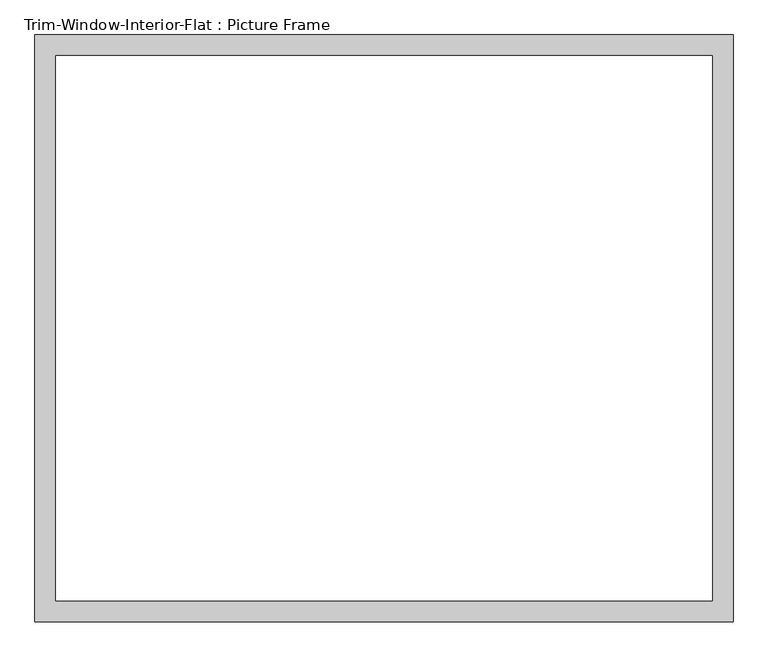
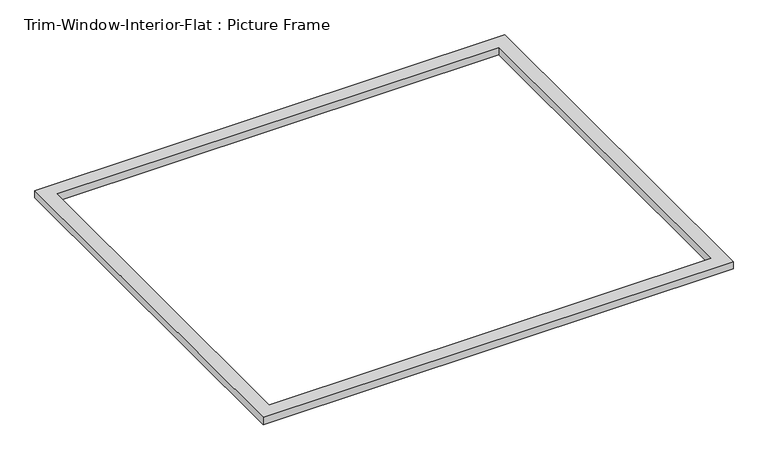
"""IFC4 building model written with IfcOpenShell, lengths in millimetres: proxy geometry, Trim-Window-Interior-Flat : Picture Frame."""

from ifc_helpers import new_model, si_unit, origin, origin_with_axes, place, context, project, spatial, polyline, outline, extrude, source, transform, mapped, element, save


def trim_window_interior_flat_picture_frame_d1f4d6ef(model_context):
    return source(origin(), model_context, "Body", "SweptSolid", [
        extrude(outline(polyline([(958.85, 44.45), (958.85, -1568.45), (-958.85, -1568.45), (-958.85, 44.45), (958.85, 44.45)]), holes=[polyline([(901.7, -12.7), (-901.7, -12.7), (-901.7, -1511.3), (901.7, -1511.3), (901.7, -12.7)])]), origin_with_axes(), (0.0, 0.0, 1.0), 31.75),
    ])


if __name__ == "__main__":
    model = new_model("IFC4")
    model_context = context("Model", 3, world=origin())
    ifc_project = project(units=[si_unit("LENGTHUNIT", "METRE", prefix="MILLI")], contexts=[model_context])
    site = spatial("IfcSite", under=ifc_project)
    building = spatial("IfcBuilding", under=site)
    placement = place(None, origin())
    trim_window_interior_flat_picture_frame_shape = trim_window_interior_flat_picture_frame_d1f4d6ef(model_context)
    element("IfcBuildingElementProxy", 1, Name="Trim-Window-Interior-Flat : Picture Frame", ObjectType="Trim-Window-Interior-Flat : Picture Frame", at=placement, inside=building, context=model_context, shape_type="MappedRepresentation", body=[
        mapped(trim_window_interior_flat_picture_frame_shape, transform((0.0, 0.0, 0.0), x_axis=(1.0, 0.0, 0.0), y_axis=(0.0, 1.0, 0.0), z_axis=(0.0, 0.0, 1.0))),
    ])
    save(model, "model.ifc")

# Revit data of these elements
# Type "Trim-Window-Interior-Flat : Picture Frame"
#   Trim Thickness_Picture Frame = 0' - 1 1/4"
#   Trim Width = 0' - 2 1/4"
#   Trim Thickness_with Sill = 0' - 0 3/4"
#   Sill Thickness = 0' - 1 1/4"
#   Opening Width [instance default] = 2' - 0"
#   Opening Height [instance default] = 3' - 0"
#   Default Elevation = 4' - 0"
#   Sill = no
#   Picture Frame = yes
#   Trim Material [instance default] = none
# Element 1 (IfcBuildingElementProxy, "Trim-Window-Interior-Flat : Picture Frame")
#   Opening Width = 6' - 0"
#   Opening Height = 5' - 0"
#   Trim Material = Wood - Stained
#   Materials on its faces: "Wood - Stained"
# Materials
#   "Wood - Stained": class "Wood", colour RGB 224 178 126, transparency 0, Cost = 0
